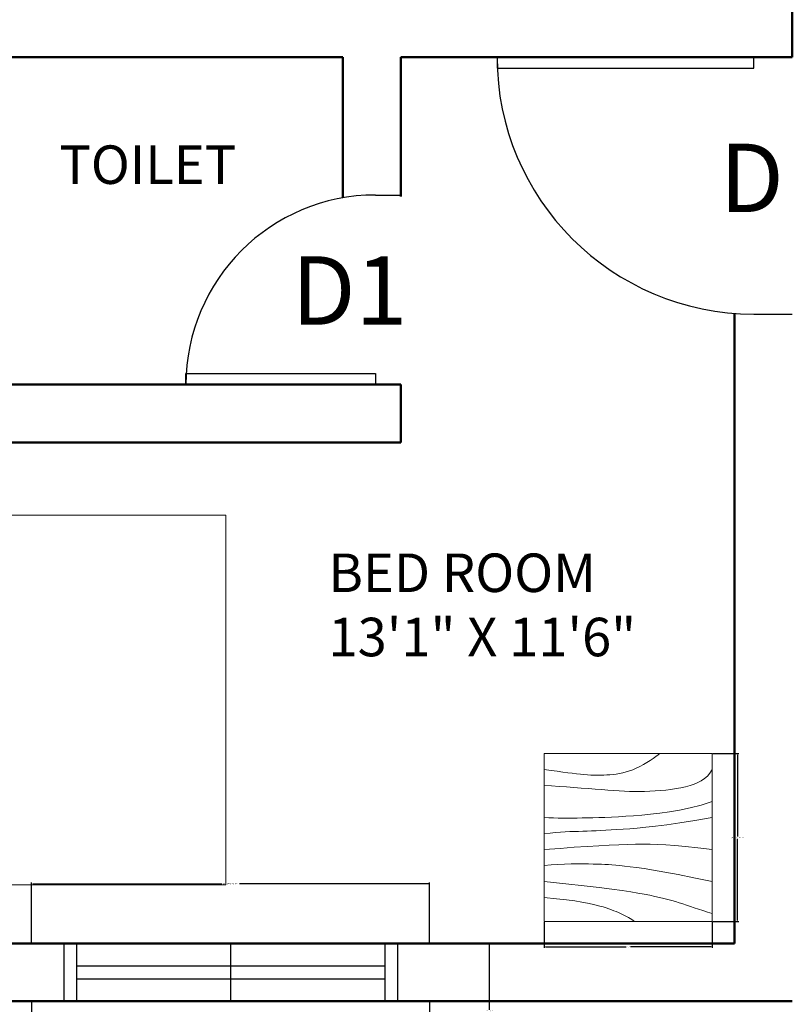
# Model space of a CAD drawing. Units: inches. Extents: x -105 to 1196, y -792 to 119.
# Tile 3 of 23: x 9 to 130, y -439 to -285. Entities that reach past the tile are written whole.
import ezdxf

# ---------------------------------------------------------------- set-up
doc = ezdxf.new("R2010")
doc.units = ezdxf.units.IN
doc.header["$MEASUREMENT"] = 0
for name, color, linetype, lineweight in [('A-ANNO-DIMS', 2, 'Continuous', 18), ('A-ANNO-TEXT', 7, 'Continuous', 25), ('A-AREA-IDEN', 7, 'Continuous', 25), ('A-DOOR', 4, 'Continuous', 25), ('A-FURN', 8, 'Continuous', 18), ('A-GLAZ', 4, 'Continuous', 25), ('A-WALL', 3, 'Continuous', 50)]:
    doc.layers.add(name, color=color, linetype=linetype, lineweight=lineweight)
doc.styles.get("Standard").update_dxf_attribs({"font": 'arial.ttf'})
doc.dimstyles.get("Standard").update_dxf_attribs({"dimtxt": 0.18, "dimasz": 0.18, "dimexe": 0.18, "dimexo": 0.0625, "dimgap": 0.09, "dimtad": 0, "dimtih": 1, "dimtoh": 1, "dimdec": 1, "dimzin": 0, "dimdsep": 46, "dimlunit": 4, "dimtxsty": 'Standard', "dimcen": 0.09, "dimadec": 0, "dimazin": 0, "dimtfac": 1, "dimtdec": 1, "dimtofl": 0, "dimtmove": 0, "dimatfit": 3, "dimfxl": 1, "dimtolj": 1, "dimtzin": 0, "dimarcsym": 0})

# ---------------------------------------------------------------- blocks, each defined once
blk = doc.blocks.new('*U17')
for p, q in [((0, 0), (0, -100)), ((750, 0), (750, -100))]:
    blk.add_line(p, q)
blk.add_lwpolyline([(0, 0), (0, 750), (43.75, 750), (43.75, 0)], close=True)
blk.add_arc((0, 0), 750, 0, 90)
blk = doc.blocks.new('Table - Square Woodgrain 42 x 42 in.')
blk.add_line((0, -42), (42, -42))
for points in [[(0, -4), (1.704, -4.2172), (3.2358, -4.4188), (4.615, -4.604), (5.8615, -4.7721), (6.9951, -4.9224), (8.0357, -5.0541), (9.0031, -5.1667), (9.9171, -5.2594), (10.7951, -5.3316), (11.6445, -5.3836), (12.4702, -5.4157), (13.277, -5.4283), (14.0698, -5.4217), (14.8535, -5.3964), (15.6331, -5.3526), (16.4133, -5.2908), (17.1986, -5.2103), (17.9913, -5.1062), (18.793, -4.9727), (19.6056, -4.8038), (20.4307, -4.5937), (21.2701, -4.3365), (22.1256, -4.0262), (22.9989, -3.6571), (23.888, -3.2272), (24.7756, -2.7516), (25.6408, -2.2491), (26.4624, -1.7387), (27.2195, -1.2395), (27.891, -0.7703), (28.456, -0.3501), (28.8934, 0.002)], [(0, -42), (0, 0), (42, 0), (42, -42)], [(0, -8), (1.8203, -8.1001), (3.6741, -8.2149), (5.5411, -8.3408), (7.4011, -8.4741), (9.2339, -8.6112), (11.0193, -8.7484), (12.7371, -8.8821), (14.3671, -9.0086), (15.8954, -9.1246), (17.3337, -9.2278), (18.6997, -9.3159), (20.0116, -9.387), (21.2871, -9.4389), (22.5442, -9.4696), (23.8008, -9.477), (25.0749, -9.459), (26.3791, -9.4137), (27.7049, -9.3403), (29.0383, -9.2382), (30.3655, -9.1068), (31.6728, -8.9455), (32.9461, -8.7535), (34.1717, -8.5304), (35.3358, -8.2756), (36.4268, -7.9863), (37.443, -7.6521), (38.3849, -7.2603), (39.253, -6.7986), (40.048, -6.2542), (40.7705, -5.6147), (41.421, -4.8674), (42, -4)], [(42, -12), (39.1784, -12.8621), (36.4519, -13.5654), (33.8246, -14.1294), (31.3004, -14.5731), (28.8832, -14.9161), (26.577, -15.1775), (24.3858, -15.3768), (22.3136, -15.5332), (20.3622, -15.6632), (18.5254, -15.7718), (16.7947, -15.8612), (15.1618, -15.9338), (13.6183, -15.9916), (12.1558, -16.0369), (10.7659, -16.0718), (9.4403, -16.0987), (8.1703, -16.1191), (6.9461, -16.1325), (5.7577, -16.1377), (4.595, -16.1335), (3.4479, -16.1188), (2.3064, -16.0924), (1.1604, -16.0532), (0, -16)], [(42, -16), (37.6529, -16.7365), (33.8802, -17.329), (30.6179, -17.7961), (27.8015, -18.1561), (25.3668, -18.4275), (23.2497, -18.6288), (21.3859, -18.7785), (19.7111, -18.8949), (18.1693, -18.9939), (16.7375, -19.0795), (15.401, -19.1534), (14.1449, -19.217), (12.9544, -19.2717), (11.8148, -19.3191), (10.7113, -19.3606), (9.6291, -19.3976), (8.5534, -19.4323), (7.47, -19.4689), (6.3643, -19.5122), (5.222, -19.5672), (4.0288, -19.6386), (2.7703, -19.7313), (1.4321, -19.8501), (0, -20)], [(0, -24), (3.9243, -23.6805), (7.4766, -23.4138), (10.6891, -23.1954), (13.5943, -23.0205), (16.2247, -22.8847), (18.6125, -22.7832), (20.7903, -22.7116), (22.7903, -22.6651), (24.6563, -22.642), (26.4764, -22.6507), (28.35, -22.7024), (30.3766, -22.8084), (32.6555, -22.98), (35.2861, -23.2283), (38.3678, -23.5645), (42, -24)], [(42, -32), (37.392, -31.017), (33.4585, -30.2231), (30.1291, -29.5949), (27.3334, -29.109), (25.0009, -28.742), (23.0612, -28.4707), (21.4439, -28.2716), (20.0786, -28.1215), (18.8998, -28.0002), (17.8609, -27.9014), (16.9206, -27.8219), (16.0371, -27.7588), (15.1691, -27.709), (14.2748, -27.6693), (13.3128, -27.6368), (12.2415, -27.6083), (11.0295, -27.5824), (9.6867, -27.5643), (8.233, -27.5608), (6.6884, -27.5787), (5.0728, -27.6248), (3.4062, -27.7058), (1.7086, -27.8286), (0, -28)], [(0, -32), (5.4026, -32.5358), (9.9494, -33.019), (13.7424, -33.4553), (16.8834, -33.8505), (19.4743, -34.2106), (21.6171, -34.5413), (23.4136, -34.8486), (24.9657, -35.1382), (26.3614, -35.4156), (27.6332, -35.6841), (28.7995, -35.9467), (29.8788, -36.2064), (30.8897, -36.4661), (31.8507, -36.7288), (32.7802, -36.9973), (33.6968, -37.2747), (34.6175, -37.5635), (35.5531, -37.8651), (36.5128, -38.1805), (37.506, -38.5108), (38.5421, -38.8568), (39.6302, -39.2197), (40.7797, -39.6004), (42, -40)], [(0, -36), (3.0098, -36.2857), (5.5354, -36.5643), (7.6368, -36.8359), (9.374, -37.1009), (10.807, -37.3597), (11.9957, -37.6126), (13.0002, -37.8599), (13.8804, -38.102), (14.6874, -38.3393), (15.4365, -38.5729), (16.1338, -38.8041), (16.7858, -39.0341), (17.3987, -39.264), (17.9787, -39.4952), (18.5322, -39.7288), (19.0655, -39.9662), (19.5832, -40.2081), (20.0842, -40.4544), (20.5657, -40.7046), (21.0249, -40.9581), (21.459, -41.2144), (21.8653, -41.4731), (22.2409, -41.7335), (22.5831, -41.9951)]]:
    blk.add_lwpolyline(points)
blk = doc.blocks.new('Bed - Queen')
for p, q in [((0, -80.00003), (0, 0)), ((0, 0), (59.99999, 0)), ((59.99999, 0), (59.99999, -80.00003)), ((7.99999, -1.2), (28.79998, -1.2)), ((7.99999, -14.4), (7.99999, -1.2)), ((28.79998, -1.2), (28.79998, -14.4)), ((31.19999, -1.2), (51.99999, -1.2)), ((31.19999, -14.4), (31.19999, -1.2)), ((51.99999, -1.2), (51.99999, -16.4)), ((0, -14.4), (44.8, -14.4)), ((59.99999, -29.6), (44.8, -14.4)), ((44.8, -14.4), (44.8, -29.6)), ((44.8, -16.8), (0, -16.8)), ((51.99999, -16.4), (46.79936, -16.4)), ((44.8, -29.6), (59.99999, -29.6)), ((59.99999, -80.00003), (0, -80.00003))]:
    blk.add_line(p, q)
blk = doc.blocks.new('*U25')
for p, q in [((0, 0), (0, -6)), ((-40, 0), (-40, -6))]:
    blk.add_line(p, q)
blk.add_lwpolyline([(0, 0), (0, 40), (-1.75, 40), (-1.75, 0)], close=True)
blk.add_arc((0, 0), 40, 90, 180)
blk = doc.blocks.new('WIN-1200')
at = {"ltscale": 2}
for p, q in [((12, 62), (0, 62)), ((0, 0), (0, 62)), ((12, 57), (12, 62)), ((12, 5), (12, 0)), ((12, 0), (0, 0))]:
    blk.add_line(p, q, dxfattribs=at)
for p, q in [((21, 57), (12, 57)), ((21, 5), (12, 5))]:
    blk.add_line(p, q)
blk = doc.blocks.new('*D55')
at = {"layer": 'A-ANNO-DIMS', "color": 0, "lineweight": -2, "transparency": 16777216}
for p, q in [((11.24, -429.16), (11.24, -419.75)), ((11.42, -419.93), (40.86, -419.93)), ((73.06, -419.93), (43.63, -419.93)), ((73.24, -429.16), (73.24, -419.75))]:
    blk.add_line(p, q, dxfattribs=at)
at = {"layer": 'A-ANNO-DIMS', "color": 0, "transparency": 16777216}
for points in [[(11.42, -419.9), (11.42, -419.96), (11.24, -419.93)], [(73.06, -419.9), (73.06, -419.96), (73.24, -419.93)]]:
    blk.add_solid(points, dxfattribs=at)
at = {"layer": 'Defpoints', "color": 0, "transparency": 16777216}
for p in [(11.24, -419.93), (11.24, -429.23), (73.24, -429.23)]:
    blk.add_point(p, dxfattribs=at)
at = {"layer": 'A-ANNO-DIMS', "color": 0, "transparency": 16777216, "insert": (42.24, -419.93), "char_height": 0.18, "attachment_point": 5}
blk.add_mtext('\\A1;WINDOW W 5\'-2" TYP.', dxfattribs=at)
blk = doc.blocks.new('*D56')
at = {"layer": 'A-ANNO-DIMS', "color": 0, "lineweight": -2, "transparency": 16777216}
for p, q in [((73.31, -429.23), (82.72, -429.23)), ((82.54, -429.41), (82.54, -439.55)), ((82.54, -450.05), (82.54, -439.91)), ((73.31, -450.23), (82.72, -450.23))]:
    blk.add_line(p, q, dxfattribs=at)
at = {"layer": 'A-ANNO-DIMS', "color": 0, "transparency": 16777216}
for points in [[(82.51, -429.41), (82.57, -429.41), (82.54, -429.23)], [(82.51, -450.05), (82.57, -450.05), (82.54, -450.23)]]:
    blk.add_solid(points, dxfattribs=at)
at = {"layer": 'Defpoints', "color": 0, "transparency": 16777216}
for p in [(73.24, -429.23), (82.54, -429.23), (73.24, -450.23)]:
    blk.add_point(p, dxfattribs=at)
at = {"layer": 'A-ANNO-DIMS', "color": 0, "transparency": 16777216, "insert": (82.54, -439.73), "char_height": 0.18, "attachment_point": 5}
blk.add_mtext('\\A1;1\'-9" TYP.', dxfattribs=at)
blk = doc.blocks.new('*D81')
at = {"layer": 'A-ANNO-DIMS', "color": 0, "lineweight": -2, "transparency": 16777216}
for p, q in [((117.34, -399.67), (121.39, -399.67)), ((121.21, -399.85), (121.21, -412.57)), ((121.21, -425.66), (121.21, -412.94)), ((117.34, -425.84), (121.39, -425.84))]:
    blk.add_line(p, q, dxfattribs=at)
at = {"layer": 'A-ANNO-DIMS', "color": 0, "transparency": 16777216}
for points in [[(121.18, -399.85), (121.24, -399.85), (121.21, -399.67)], [(121.18, -425.66), (121.24, -425.66), (121.21, -425.84)]]:
    blk.add_solid(points, dxfattribs=at)
at = {"layer": 'Defpoints', "color": 0, "transparency": 16777216}
for p in [(117.28, -399.67), (121.21, -399.67), (117.28, -425.84)]:
    blk.add_point(p, dxfattribs=at)
at = {"layer": 'A-ANNO-DIMS', "color": 0, "transparency": 16777216, "insert": (121.21, -412.75), "char_height": 0.18, "attachment_point": 5}
blk.add_mtext('\\A1;SIDE TABLE 2\'-2"', dxfattribs=at)
blk = doc.blocks.new('*D82')
at = {"layer": 'A-ANNO-DIMS', "color": 0, "lineweight": -2, "transparency": 16777216}
for p, q in [((91.11, -425.9), (91.11, -429.94)), ((117.28, -425.9), (117.28, -429.94)), ((91.29, -429.76), (103.87, -429.76)), ((117.1, -429.76), (104.53, -429.76))]:
    blk.add_line(p, q, dxfattribs=at)
at = {"layer": 'A-ANNO-DIMS', "color": 0, "transparency": 16777216}
for points in [[(91.29, -429.73), (91.29, -429.79), (91.11, -429.76)], [(117.1, -429.73), (117.1, -429.79), (117.28, -429.76)]]:
    blk.add_solid(points, dxfattribs=at)
at = {"layer": 'Defpoints', "color": 0, "transparency": 16777216}
for p in [(91.11, -425.84), (117.28, -425.84), (117.28, -429.76)]:
    blk.add_point(p, dxfattribs=at)
at = {"layer": 'A-ANNO-DIMS', "color": 0, "transparency": 16777216, "insert": (104.2, -429.76), "char_height": 0.18, "attachment_point": 5}
blk.add_mtext('\\A1;2\'-2"', dxfattribs=at)

msp = doc.modelspace()

# ---------------------------------------------------------------- linework, layer by layer
at = {"layer": 'A-GLAZ'}
for p, q in [((18.24, -429.23), (18.24, -438.23)), ((42.24, -429.23), (42.24, -438.23)), ((66.24, -429.23), (66.24, -438.23)), ((18.24, -432.73), (66.24, -432.73)), ((18.24, -434.73), (66.24, -434.73))]:
    msp.add_line(p, q, dxfattribs=at)
at = {"layer": 'A-WALL'}
for p, q in [((129.74, -282.23), (129.74, -291.23)), ((-36.26, -291.23), (59.74, -291.23)), ((59.74, -313.14), (59.74, -291.23)), ((68.74, -291.23), (129.74, -291.23)), ((68.74, -312.96), (68.74, -291.23)), ((120.74, -429.23), (120.74, -331.11)), ((-36.26, -342.23), (68.74, -342.23)), ((68.74, -351.23), (68.74, -342.23)), ((-36.26, -351.23), (68.74, -351.23)), ((-36.26, -429.23), (120.74, -429.23)), ((-45.26, -438.23), (129.74, -438.23))]:
    msp.add_line(p, q, dxfattribs=at)

# ---------------------------------------------------------------- block references
at = {"layer": 'A-DOOR', "rotation": 90}
msp.add_blockref('*U25', (123.74, -291.23), dxfattribs=at)
at = {"layer": 'A-DOOR', "xscale": 0.0393700787401575, "yscale": 0.0393700787401575, "zscale": 0.0393700787401575, "rotation": 89.99999999999999}
msp.add_blockref('*U17', (64.81, -342.23), dxfattribs=at)
at = {"layer": 'A-FURN', "xscale": 0.9593862173514477, "yscale": 0.9593862173514477, "zscale": 0.9593862173514477, "rotation": 90}
msp.add_blockref('Bed - Queen', (-35.26, -420.11), dxfattribs=at)
at = {"layer": 'A-FURN', "xscale": 0.6230052676484834, "yscale": 0.6230052676484834, "zscale": 0.6230052676484834}
msp.add_blockref('Table - Square Woodgrain 42 x 42 in.', (91.11, -399.67), dxfattribs=at)
at = {"layer": 'A-GLAZ', "rotation": 90.00000000000006}
msp.add_blockref('WIN-1200', (73.24, -450.23), dxfattribs=at)

# ---------------------------------------------------------------- texts
at = {"layer": 'A-ANNO-TEXT'}
for s, height, p in [('D', 10.64, (118.43, -315.36)), ('D1', 10.636, (51.72, -332.89))]:
    msp.add_text(s, height=height, dxfattribs=at).set_placement(p)
at = {"layer": 'A-AREA-IDEN', "char_height": 6, "attachment_point": 1}
for s, insert in [('TOILET', (15.56, -304.98)), ('BED ROOM\\P13\'1" X 11\'6"', (57.48, -368.52))]:
    msp.add_mtext_dynamic_manual_height_columns(s, width=59.5623, gutter_width=1, heights=[0], dxfattribs=dict(at, insert=insert))

# ---------------------------------------------------------------- dimensions: what is measured, and where the dimension line sits
at = {"layer": 'A-ANNO-DIMS'}
for base, p1, p2, angle, text, picture, middle in [((121.21, -399.67), (117.28, -425.84), (117.28, -399.67), 90, 'SIDE TABLE <>', '*D81', (121.21, -412.75)), ((11.24, -419.93), (73.24, -429.23), (11.24, -429.23), 180, 'WINDOW W <> TYP.', '*D55', (42.24, -419.93)), ((82.54, -429.23), (73.24, -450.23), (73.24, -429.23), 90, '<> TYP.', '*D56', (82.54, -439.73))]:
    dim = msp.add_linear_dim(base=base, p1=p1, p2=p2, angle=angle, text=text, dimstyle='Standard', override={"dimdec": 1, "dimlfac": 1, "dimrnd": 0, "dimzin": 1, "dimdsep": 46, "dimlunit": 4, "dimfrac": 2}, dxfattribs=at)
    dim.commit()
    dim.dimension.update_dxf_attribs({"geometry": picture, "text_midpoint": middle})
dim = msp.add_linear_dim(base=(117.28, -429.76), p1=(91.11, -425.84), p2=(117.28, -425.84), dimstyle='Standard', override={"dimdec": 1, "dimlfac": 1, "dimrnd": 0, "dimzin": 1, "dimdsep": 46, "dimlunit": 4, "dimfrac": 2}, dxfattribs=at)
dim.commit()
dim.dimension.update_dxf_attribs({"geometry": '*D82', "text_midpoint": (104.2, -429.76)})

doc.saveas('drawing.dxf')
